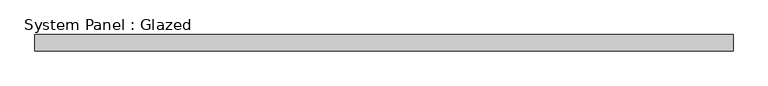
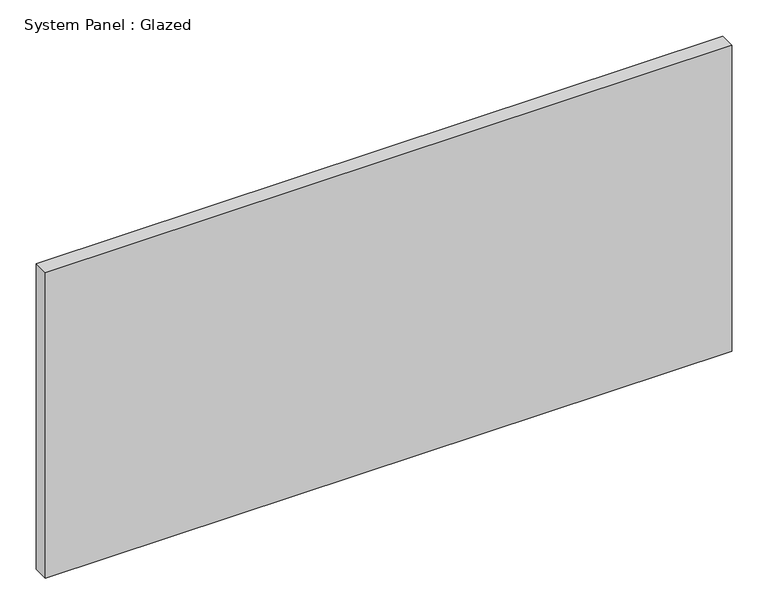
"""IFC4 building model written with IfcOpenShell, lengths in millimetres: plate geometry, System Panel : Glazed."""

from ifc_helpers import new_model, si_unit, origin, origin_with_axes, place, context, project, spatial, polyline, outline, extrude, source, transform, mapped, element, save


def system_panel_glazed_3290db12(model_context):
    return source(origin(), model_context, "Body", "SweptSolid", [
        extrude(outline(polyline([(546.1, 19.05), (-546.1, 19.05), (-546.1, 44.45), (546.1, 44.45), (546.1, 19.05)])), origin_with_axes(), (0.0, 0.0, 1.0), 514.35),
    ])


if __name__ == "__main__":
    model = new_model("IFC4")
    model_context = context("Model", 3, world=origin())
    ifc_project = project(units=[si_unit("LENGTHUNIT", "METRE", prefix="MILLI")], contexts=[model_context])
    site = spatial("IfcSite", under=ifc_project)
    building = spatial("IfcBuilding", under=site)
    placement = place(None, origin())
    system_panel_glazed_shape = system_panel_glazed_3290db12(model_context)
    element("IfcPlate", 1, ObjectType="System Panel : Glazed", at=placement, inside=building, context=model_context, shape_type="MappedRepresentation", body=[
        mapped(system_panel_glazed_shape, transform((0.0, 0.0, 0.0), x_axis=(1.0, 0.0, 0.0), y_axis=(0.0, 1.0, 0.0), z_axis=(0.0, 0.0, 1.0))),
    ])
    save(model, "model.ifc")

# Revit data of these elements
# Type "System Panel : Glazed"
#   Construction Type Id = "GSP4R"
#   Analytic Construction = "1/8 in Pilkington single glazing"
#   Visual Light Transmittance = 0.9
#   Solar Heat Gain Coefficient = 0.86
#   Heat Transfer Coefficient (U) = 1.18115 BTU/(h·ft²·°F)
#   Define Thermal Properties by = 1
# Element 1 (IfcPlate, "System Panel : Glazed")
#   Materials on its faces: "Glass"
# Materials
#   "Glass": class "Glass", colour RGB 0 128 192, transparency 0.75, Description = "Soda Lime Glass", Cost = 0
